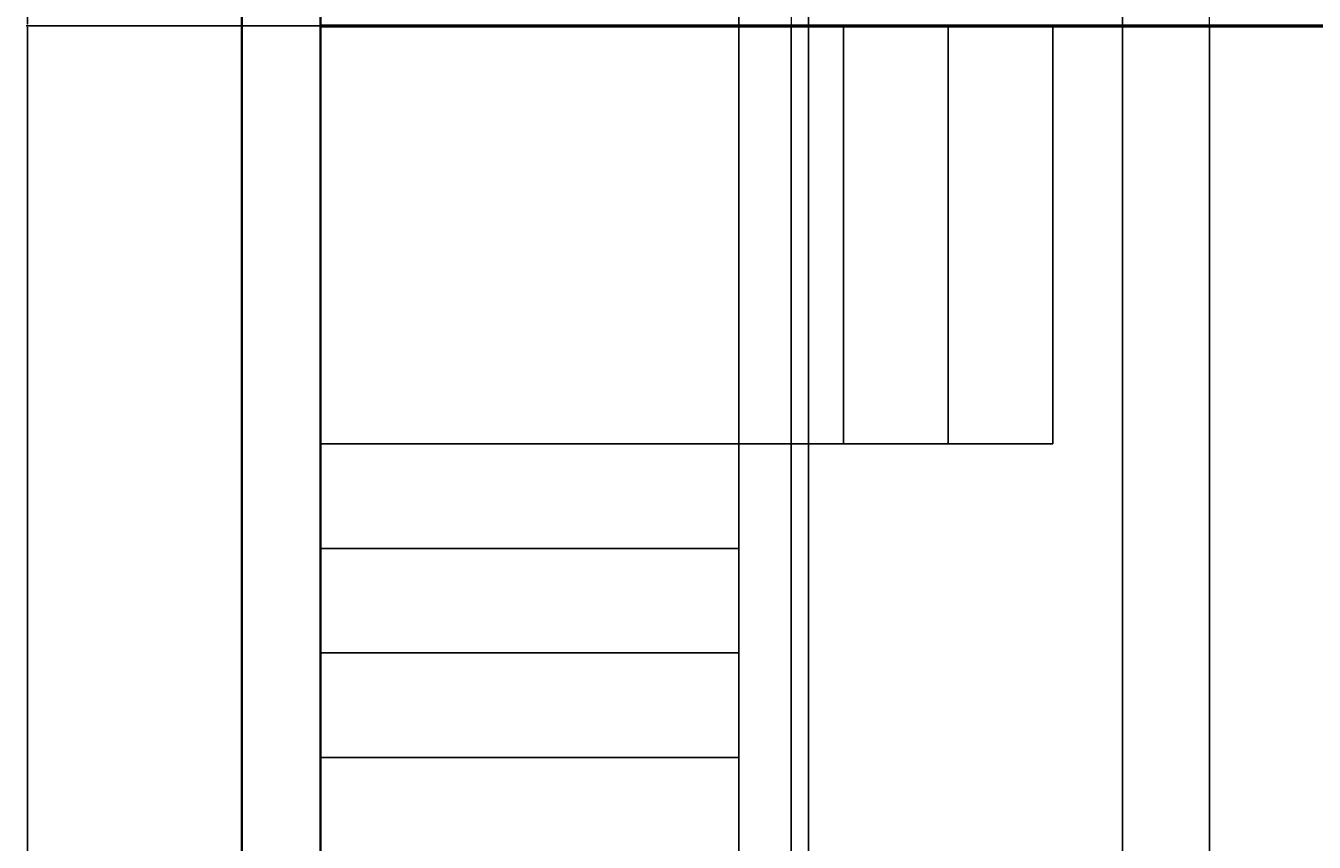
# Model space of a CAD drawing. Units: inches. Extents: x 8049 to 8459, y 820 to 1350.
# Tile 18 of 25: x 8050 to 8197, y 952 to 1046. Entities that reach past the tile are written whole.
import ezdxf

# ---------------------------------------------------------------- set-up
doc = ezdxf.new("R2010")
doc.units = ezdxf.units.IN
doc.header["$MEASUREMENT"] = 0
for name, color, linetype, lineweight in [('A-ANNO-DIMS', 2, 'Continuous', 18), ('A-FLOR-STRS', 7, 'Continuous', 25), ('A-GLAZ', 4, 'Continuous', 18), ('A-WALL', 7, 'Continuous', 50), ('C-SITE-WALL', 7, 'Continuous', 35)]:
    doc.layers.add(name, color=color, linetype=linetype, lineweight=lineweight)
doc.styles.get("Standard").update_dxf_attribs({"font": 'arial.ttf'})
doc.dimstyles.get("Standard").update_dxf_attribs({"dimtxt": 0.18, "dimasz": 0.18, "dimexe": 0.18, "dimexo": 0.0625, "dimgap": 0.09, "dimtad": 0, "dimtih": 1, "dimtoh": 1, "dimdec": 4, "dimzin": 0, "dimdsep": 46, "dimtxsty": 'Standard', "dimcen": 0.09, "dimadec": 0, "dimazin": 0, "dimtfac": 1, "dimtdec": 4, "dimtofl": 0, "dimtmove": 0, "dimatfit": 3, "dimfxl": 1, "dimtolj": 1, "dimtzin": 0, "dimarcsym": 0})

# ---------------------------------------------------------------- blocks, each defined once
blk = doc.blocks.new('WIN-48IN-SURROUND')
for p, q in [((9, 48), (0, 48)), ((0, 48), (0, 0)), ((0, 0), (9, 0))]:
    blk.add_line(p, q)
blk = doc.blocks.new('*D50')
at = {"layer": 'A-ANNO-DIMS', "color": 0, "lineweight": -2, "transparency": 16777216}
for p, q in [((8083.33, 1045.87), (8049.62, 1045.87)), ((8049.8, 1045.69), (8049.8, 945.55)), ((8049.8, 845.05), (8049.8, 945.19)), ((8074.33, 844.87), (8049.62, 844.87))]:
    blk.add_line(p, q, dxfattribs=at)
at = {"layer": 'A-ANNO-DIMS', "color": 0, "transparency": 16777216}
for points in [[(8049.77, 1045.69), (8049.83, 1045.69), (8049.8, 1045.87)], [(8049.77, 845.05), (8049.83, 845.05), (8049.8, 844.87)]]:
    blk.add_solid(points, dxfattribs=at)
at = {"layer": 'Defpoints', "color": 0, "transparency": 16777216}
for p in [(8049.8, 1045.87), (8083.4, 1045.87), (8074.4, 844.87)]:
    blk.add_point(p, dxfattribs=at)
at = {"layer": 'A-ANNO-DIMS', "color": 0, "transparency": 16777216, "insert": (8049.8, 945.37), "char_height": 0.18, "attachment_point": 5}
blk.add_mtext('\\A1;201', dxfattribs=at)
blk = doc.blocks.new('*D51')
at = {"layer": 'A-ANNO-DIMS', "color": 0, "lineweight": -2, "transparency": 16777216}
for p, q in [((8083.33, 1267.87), (8049.62, 1267.87)), ((8049.8, 1267.69), (8049.8, 1157.05)), ((8049.8, 1046.05), (8049.8, 1156.69)), ((8083.33, 1045.87), (8049.62, 1045.87))]:
    blk.add_line(p, q, dxfattribs=at)
at = {"layer": 'A-ANNO-DIMS', "color": 0, "transparency": 16777216}
for points in [[(8049.77, 1267.69), (8049.83, 1267.69), (8049.8, 1267.87)], [(8049.77, 1046.05), (8049.83, 1046.05), (8049.8, 1045.87)]]:
    blk.add_solid(points, dxfattribs=at)
at = {"layer": 'Defpoints', "color": 0, "transparency": 16777216}
for p in [(8049.8, 1267.87), (8083.4, 1267.87), (8083.4, 1045.87)]:
    blk.add_point(p, dxfattribs=at)
at = {"layer": 'A-ANNO-DIMS', "color": 0, "transparency": 16777216, "insert": (8049.8, 1156.87), "char_height": 0.18, "attachment_point": 5}
blk.add_mtext('\\A1;222', dxfattribs=at)
blk = doc.blocks.new('*D58')
at = {"layer": 'A-ANNO-DIMS', "color": 0, "lineweight": -2, "transparency": 16777216}
for p, q in [((8139.4, 1162.81), (8139.4, 820.09)), ((8175.4, 1162.81), (8175.4, 820.09)), ((8139.58, 820.27), (8157.18, 820.27)), ((8175.22, 820.27), (8157.62, 820.27))]:
    blk.add_line(p, q, dxfattribs=at)
at = {"layer": 'A-ANNO-DIMS', "color": 0, "transparency": 16777216}
for points in [[(8139.58, 820.3), (8139.58, 820.24), (8139.4, 820.27)], [(8175.22, 820.3), (8175.22, 820.24), (8175.4, 820.27)]]:
    blk.add_solid(points, dxfattribs=at)
at = {"layer": 'Defpoints', "color": 0, "transparency": 16777216}
for p in [(8139.4, 1162.87), (8175.4, 1162.87), (8175.4, 820.27)]:
    blk.add_point(p, dxfattribs=at)
at = {"layer": 'A-ANNO-DIMS', "color": 0, "transparency": 16777216, "insert": (8157.4, 820.27), "char_height": 0.18, "attachment_point": 5}
blk.add_mtext('\\A1;36', dxfattribs=at)
blk = doc.blocks.new('*D59')
at = {"layer": 'A-ANNO-DIMS', "color": 0, "lineweight": -2, "transparency": 16777216}
for p, q in [((8083.4, 925.93), (8083.4, 1349.65)), ((8083.58, 1349.47), (8107.17, 1349.47)), ((8131.22, 1349.47), (8107.62, 1349.47)), ((8131.4, 925.93), (8131.4, 1349.65))]:
    blk.add_line(p, q, dxfattribs=at)
at = {"layer": 'A-ANNO-DIMS', "color": 0, "transparency": 16777216}
for points in [[(8083.58, 1349.5), (8083.58, 1349.44), (8083.4, 1349.47)], [(8131.22, 1349.5), (8131.22, 1349.44), (8131.4, 1349.47)]]:
    blk.add_solid(points, dxfattribs=at)
at = {"layer": 'Defpoints', "color": 0, "transparency": 16777216}
for p in [(8131.4, 1349.47), (8083.4, 925.87), (8131.4, 925.87)]:
    blk.add_point(p, dxfattribs=at)
at = {"layer": 'A-ANNO-DIMS', "color": 0, "transparency": 16777216, "insert": (8107.4, 1349.47), "char_height": 0.18, "attachment_point": 5}
blk.add_mtext('\\A1;48', dxfattribs=at)
blk = doc.blocks.new('*D70')
at = {"layer": 'A-ANNO-DIMS', "color": 0, "lineweight": -2, "transparency": 16777216}
for p, q in [((8083.4, 1045.81), (8083.4, 820.09)), ((8137.4, 1045.81), (8137.4, 820.09)), ((8083.58, 820.27), (8110.18, 820.27)), ((8137.22, 820.27), (8110.62, 820.27))]:
    blk.add_line(p, q, dxfattribs=at)
at = {"layer": 'A-ANNO-DIMS', "color": 0, "transparency": 16777216}
for points in [[(8083.58, 820.3), (8083.58, 820.24), (8083.4, 820.27)], [(8137.22, 820.3), (8137.22, 820.24), (8137.4, 820.27)]]:
    blk.add_solid(points, dxfattribs=at)
at = {"layer": 'Defpoints', "color": 0, "transparency": 16777216}
for p in [(8083.4, 1045.87), (8137.4, 1045.87), (8083.4, 820.27)]:
    blk.add_point(p, dxfattribs=at)
at = {"layer": 'A-ANNO-DIMS', "color": 0, "transparency": 16777216, "insert": (8110.4, 820.27), "char_height": 0.18, "attachment_point": 5}
blk.add_mtext('\\A1;54', dxfattribs=at)
blk = doc.blocks.new('*D71')
at = {"layer": 'A-ANNO-DIMS', "color": 0, "lineweight": -2, "transparency": 16777216}
for p, q in [((8185.4, 1045.81), (8185.4, 820.09)), ((8239.4, 1045.81), (8239.4, 820.09)), ((8185.58, 820.27), (8212.18, 820.27)), ((8239.22, 820.27), (8212.62, 820.27))]:
    blk.add_line(p, q, dxfattribs=at)
at = {"layer": 'A-ANNO-DIMS', "color": 0, "transparency": 16777216}
for points in [[(8185.58, 820.3), (8185.58, 820.24), (8185.4, 820.27)], [(8239.22, 820.3), (8239.22, 820.24), (8239.4, 820.27)]]:
    blk.add_solid(points, dxfattribs=at)
at = {"layer": 'Defpoints', "color": 0, "transparency": 16777216}
for p in [(8185.4, 1045.87), (8239.4, 1045.87), (8239.4, 820.27)]:
    blk.add_point(p, dxfattribs=at)
at = {"layer": 'A-ANNO-DIMS', "color": 0, "transparency": 16777216, "insert": (8212.4, 820.27), "char_height": 0.18, "attachment_point": 5}
blk.add_mtext('\\A1;54', dxfattribs=at)
blk = doc.blocks.new('*D76')
at = {"layer": 'A-ANNO-DIMS', "color": 0, "lineweight": -2, "transparency": 16777216}
for p, q in [((8083.4, 1054.81), (8083.4, 820.09)), ((8299.4, 1054.81), (8299.4, 820.09)), ((8083.58, 820.27), (8191.11, 820.27)), ((8299.22, 820.27), (8191.69, 820.27))]:
    blk.add_line(p, q, dxfattribs=at)
at = {"layer": 'A-ANNO-DIMS', "color": 0, "transparency": 16777216}
for points in [[(8083.58, 820.3), (8083.58, 820.24), (8083.4, 820.27)], [(8299.22, 820.3), (8299.22, 820.24), (8299.4, 820.27)]]:
    blk.add_solid(points, dxfattribs=at)
at = {"layer": 'Defpoints', "color": 0, "transparency": 16777216}
for p in [(8083.4, 1054.87), (8299.4, 1054.87), (8299.4, 820.27)]:
    blk.add_point(p, dxfattribs=at)
at = {"layer": 'A-ANNO-DIMS', "color": 0, "transparency": 16777216, "insert": (8191.4, 820.27), "char_height": 0.18, "attachment_point": 5}
blk.add_mtext('\\A1;216', dxfattribs=at)
blk = doc.blocks.new('*D88')
at = {"layer": 'A-ANNO-DIMS', "color": 0, "lineweight": -2, "transparency": 16777216}
for p, q in [((8083.4, 1162.81), (8083.4, 820.09)), ((8139.4, 1162.81), (8139.4, 820.09)), ((8083.58, 820.27), (8111.18, 820.27)), ((8139.22, 820.27), (8111.62, 820.27))]:
    blk.add_line(p, q, dxfattribs=at)
at = {"layer": 'A-ANNO-DIMS', "color": 0, "transparency": 16777216}
for points in [[(8083.58, 820.3), (8083.58, 820.24), (8083.4, 820.27)], [(8139.22, 820.3), (8139.22, 820.24), (8139.4, 820.27)]]:
    blk.add_solid(points, dxfattribs=at)
at = {"layer": 'Defpoints', "color": 0, "transparency": 16777216}
for p in [(8083.4, 1162.87), (8139.4, 1162.87), (8139.4, 820.27)]:
    blk.add_point(p, dxfattribs=at)
at = {"layer": 'A-ANNO-DIMS', "color": 0, "transparency": 16777216, "insert": (8111.4, 820.27), "char_height": 0.18, "attachment_point": 5}
blk.add_mtext('\\A1;56', dxfattribs=at)

msp = doc.modelspace()

# ---------------------------------------------------------------- linework, layer by layer
at = {"layer": 'A-FLOR-STRS'}
for p, q in [((8131.3974, 1045.8706), (8131.3974, 925.8706)), ((8143.3974, 1045.8706), (8143.3974, 997.8706)), ((8155.3974, 1045.8706), (8155.3974, 997.8706)), ((8167.3974, 1045.8706), (8167.3974, 997.8706)), ((8083.3974, 997.8706), (8167.3974, 997.8706)), ((8083.3974, 985.8706), (8131.3974, 985.8706)), ((8083.3974, 973.8706), (8131.3974, 973.8706)), ((8083.3974, 961.8706), (8131.3974, 961.8706))]:
    msp.add_line(p, q, dxfattribs=at)
at = {"layer": 'A-WALL'}
msp.add_line((8083.3974, 1045.8706), (8239.3974, 1045.8706), dxfattribs=at)
at = {"layer": 'C-SITE-WALL'}
for p, q in [((8074.3974, 1324.8706), (8074.3974, 844.8706)), ((8083.3974, 1315.8706), (8083.3974, 853.8706))]:
    msp.add_line(p, q, dxfattribs=at)

# ---------------------------------------------------------------- block references
at = {"layer": 'A-GLAZ', "rotation": 89.9999999999985}
msp.add_blockref('WIN-48IN-SURROUND', (8185.397, 1045.8702), dxfattribs=at)

# ---------------------------------------------------------------- dimensions: what is measured, and where the dimension line sits
at = {"layer": 'A-ANNO-DIMS'}
for base, p1, p2, picture, middle in [((8131.3974, 1349.4706), (8083.3974, 925.8706), (8131.3974, 925.8706), '*D59', (8107.3974, 1349.4706)), ((8139.3974, 820.2706), (8083.3974, 1162.8706), (8139.3974, 1162.8706), '*D88', (8111.3974, 820.2706)), ((8175.3974, 820.2706), (8139.3974, 1162.8706), (8175.3974, 1162.8706), '*D58', (8157.3974, 820.2706)), ((8299.3974, 820.2706), (8083.3974, 1054.8706), (8299.3974, 1054.8706), '*D76', (8191.3974, 820.2706)), ((8083.3974, 820.2706), (8137.3974, 1045.8706), (8083.3974, 1045.8706), '*D70', (8110.3974, 820.2706)), ((8239.3974, 820.2706), (8185.3974, 1045.8706), (8239.3974, 1045.8706), '*D71', (8212.3974, 820.2706))]:
    dim = msp.add_linear_dim(base=base, p1=p1, p2=p2, dimstyle='Standard', override={"dimdec": 0, "dimlfac": 1, "dimrnd": 0, "dimzin": 0, "dimdsep": 46, "dimlunit": 2}, dxfattribs=at)
    dim.commit()
    dim.dimension.update_dxf_attribs({"geometry": picture, "text_midpoint": middle})
for base, p1, p2, picture, middle in [((8049.7974, 1267.8706), (8083.3974, 1045.8706), (8083.3974, 1267.8706), '*D51', (8049.7974, 1156.8706)), ((8049.7974, 1045.8706), (8074.3974, 844.8706), (8083.3974, 1045.8706), '*D50', (8049.7974, 945.3706))]:
    dim = msp.add_linear_dim(base=base, p1=p1, p2=p2, angle=90, dimstyle='Standard', override={"dimdec": 0, "dimlfac": 1, "dimrnd": 0, "dimzin": 0, "dimdsep": 46, "dimlunit": 2}, dxfattribs=at)
    dim.commit()
    dim.dimension.update_dxf_attribs({"geometry": picture, "text_midpoint": middle})

doc.saveas('drawing.dxf')
